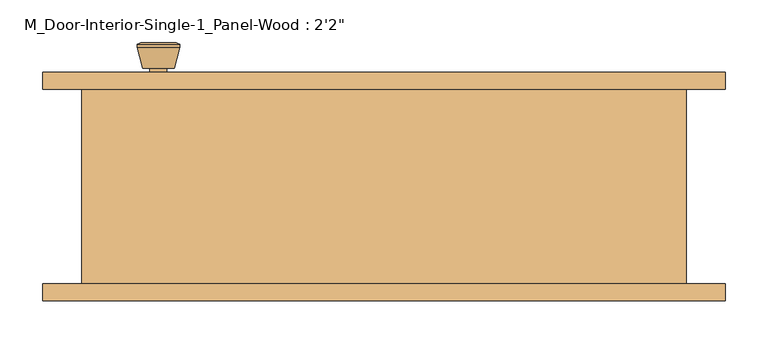
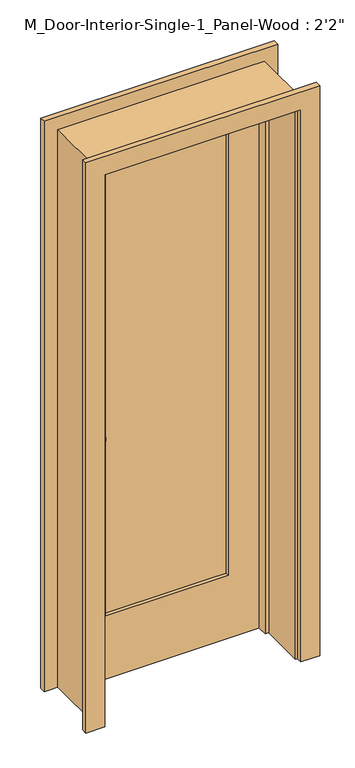
"""IFC4 building model written with IfcOpenShell, lengths in millimetres: door geometry."""

from ifc_helpers import new_model, si_unit, point, frame, frame_2d, origin, place, context, project, spatial, polyline, circle_curve, trimmed, segment, composite_curve, outline, extrude, faceted_brep, source, transform, mapped, element, save
from ifc_brep_helpers import plane_surface, cylinder_surface, revolved_surface, advanced_brep


def door_ae2d502c(model_context):
    return source(origin(), model_context, "Body", "SolidModel", [
        advanced_brep(
        [(-265.2, 70.125, 914.4), (-255.2, 70.125, 914.4), (-275.2, 70.125, 914.4), (-244.7241324, 21.125, 914.4), (-265.2, 21.125, 914.4), (-285.6758676, 21.125, 914.4), (-240.2, 22.9528681, 914.4), (-290.2, 22.9528681, 914.4), (-240.2, 26.4165463, 914.4), (-290.2, 26.4165463, 914.4), (-246.563764, 51.125, 914.4), (-283.836236, 51.125, 914.4), (-255.2, 51.125, 914.4), (-275.2, 51.125, 914.4)],
        [
            (0, 1),
            (1, 2, circle_curve(frame((-265.2, 70.125, 914.4), z_axis=(0.0, 1.0, 0.0), x_axis=(-1.0, 0.0, 0.0)), 10.0)),
            (2, 0),
            (2, 1, circle_curve(frame((-265.2, 70.125, 914.4), z_axis=(0.0, 1.0, 0.0), x_axis=(-1.0, 0.0, 0.0)), 10.0)),
            (3, 4),
            (4, 5),
            (5, 3, circle_curve(frame((-265.2, 21.125, 914.4), z_axis=(0.0, -1.0, 0.0), x_axis=(-1.0, 0.0, 0.0)), 20.4758676)),
            (3, 5, circle_curve(frame((-265.2, 21.125, 914.4), z_axis=(0.0, -1.0, 0.0), x_axis=(-1.0, 0.0, 0.0)), 20.4758676)),
            (6, 3),
            (5, 7),
            (7, 6, circle_curve(frame((-265.2, 22.9528681, 914.4), z_axis=(0.0, -1.0, 0.0), x_axis=(-1.0, 0.0, 0.0)), 25.0)),
            (6, 7, circle_curve(frame((-265.2, 22.9528681, 914.4), z_axis=(0.0, -1.0, 0.0), x_axis=(-1.0, 0.0, 0.0)), 25.0)),
            (8, 6),
            (7, 9),
            (9, 8, circle_curve(frame((-265.2, 26.4165463, 914.4), z_axis=(0.0, -1.0, 0.0), x_axis=(-1.0, 0.0, 0.0)), 25.0)),
            (8, 9, circle_curve(frame((-265.2, 26.4165463, 914.4), z_axis=(0.0, -1.0, 0.0), x_axis=(-1.0, 0.0, 0.0)), 25.0)),
            (10, 8),
            (9, 11),
            (11, 10, circle_curve(frame((-265.2, 51.125, 914.4), z_axis=(0.0, -1.0, 0.0), x_axis=(-1.0, 0.0, 0.0)), 18.636236)),
            (10, 11, circle_curve(frame((-265.2, 51.125, 914.4), z_axis=(0.0, -1.0, 0.0), x_axis=(-1.0, 0.0, 0.0)), 18.636236)),
            (12, 10),
            (11, 13),
            (13, 12, circle_curve(frame((-265.2, 51.125, 914.4), z_axis=(0.0, -1.0, 0.0), x_axis=(-1.0, 0.0, 0.0)), 10.0)),
            (12, 13, circle_curve(frame((-265.2, 51.125, 914.4), z_axis=(0.0, -1.0, 0.0), x_axis=(-1.0, 0.0, 0.0)), 10.0)),
            (1, 12),
            (13, 2),
        ],
        [
            plane_surface(frame((-265.2, 70.125, 914.4), z_axis=(0.0, 1.0, 0.0), x_axis=(-1.0, 0.0, 0.0))),
            plane_surface(frame((-265.2, 21.125, 914.4), z_axis=(0.0, -1.0, 0.0), x_axis=(-1.0, 0.0, 0.0))),
            revolved_surface(polyline([(-285.6758676, 21.125, 914.4), (-290.2, 22.9528681, 914.4)]), (-265.2, 70.125, 914.4), (0.0, 1.0, 0.0)),
            cylinder_surface(frame((-265.2, 70.125, 914.4), z_axis=(0.0, 1.0, 0.0), x_axis=(-1.0, 0.0, 0.0)), 25.0),
            revolved_surface(polyline([(-290.2, 26.4165463, 914.4), (-283.836236, 51.125, 914.4)]), (-265.2, 70.125, 914.4), (0.0, 1.0, 0.0)),
            plane_surface(frame((-265.2, 51.125, 914.4), z_axis=(0.0, 1.0, 0.0), x_axis=(-1.0, 0.0, 0.0))),
            cylinder_surface(frame((-265.2, 70.125, 914.4), z_axis=(0.0, 1.0, 0.0), x_axis=(-1.0, 0.0, 0.0)), 10.0),
        ],
        [
            (0, [[1, 2, 3]]),
            (0, [[-3, 4, -1]]),
            (1, [[5, 6, 7]]),
            (1, [[-6, -5, 8]]),
            (2, [[9, -7, 10, 11]]),
            (2, [[-10, -8, -9, 12]]),
            (3, [[13, -11, 14, 15]]),
            (3, [[-14, -12, -13, 16]]),
            (4, [[17, -15, 18, 19]]),
            (4, [[-18, -16, -17, 20]]),
            (5, [[21, -19, 22, 23]]),
            (5, [[-22, -20, -21, 24]]),
            (6, [[25, -23, 26, -2]]),
            (6, [[-26, -24, -25, -4]]),
        ],
    ),
        extrude(outline(composite_curve([segment(trimmed(circle_curve(frame_2d((914.4, -265.2)), 30.0), [point((914.4, -295.2))], [point((914.4, -235.2))], False, "CARTESIAN"), True, "CONTINUOUS"), segment(trimmed(circle_curve(frame_2d((914.4, -265.2)), 30.0), [point((914.4, -235.2))], [point((914.4, -295.2))], False, "CARTESIAN"), True, "CONTINUOUS")], self_intersect=False)), frame((0.0, 70.125, 0.0), z_axis=(0.0, 1.0, 0.0), x_axis=(0.0, 0.0, 1.0)), (0.0, 0.0, 1.0), 6.0),
        advanced_brep(
        [(-265.2, 117.125, 914.4), (-275.2, 117.125, 914.4), (-255.2, 117.125, 914.4), (-244.7241324, 166.125, 914.4), (-285.6758676, 166.125, 914.4), (-265.2, 166.125, 914.4), (-240.2, 164.2971319, 914.4), (-290.2, 164.2971319, 914.4), (-240.2, 160.8334537, 914.4), (-290.2, 160.8334537, 914.4), (-246.563764, 136.125, 914.4), (-283.836236, 136.125, 914.4), (-255.2, 136.125, 914.4), (-275.2, 136.125, 914.4)],
        [
            (0, 1),
            (1, 2, circle_curve(frame((-265.2, 117.125, 914.4), z_axis=(0.0, -1.0, 0.0), x_axis=(-1.0, 0.0, 0.0)), 10.0)),
            (2, 0),
            (2, 1, circle_curve(frame((-265.2, 117.125, 914.4), z_axis=(0.0, -1.0, 0.0), x_axis=(-1.0, 0.0, 0.0)), 10.0)),
            (3, 4, circle_curve(frame((-265.2, 166.125, 914.4), z_axis=(0.0, 1.0, 0.0), x_axis=(-1.0, 0.0, 0.0)), 20.4758676)),
            (4, 5),
            (5, 3),
            (4, 3, circle_curve(frame((-265.2, 166.125, 914.4), z_axis=(0.0, 1.0, 0.0), x_axis=(-1.0, 0.0, 0.0)), 20.4758676)),
            (6, 7, circle_curve(frame((-265.2, 164.2971319, 914.4), z_axis=(0.0, 1.0, 0.0), x_axis=(-1.0, 0.0, 0.0)), 25.0)),
            (7, 4),
            (3, 6),
            (7, 6, circle_curve(frame((-265.2, 164.2971319, 914.4), z_axis=(0.0, 1.0, 0.0), x_axis=(-1.0, 0.0, 0.0)), 25.0)),
            (8, 9, circle_curve(frame((-265.2, 160.8334537, 914.4), z_axis=(0.0, 1.0, 0.0), x_axis=(-1.0, 0.0, 0.0)), 25.0)),
            (9, 7),
            (6, 8),
            (9, 8, circle_curve(frame((-265.2, 160.8334537, 914.4), z_axis=(0.0, 1.0, 0.0), x_axis=(-1.0, 0.0, 0.0)), 25.0)),
            (10, 11, circle_curve(frame((-265.2, 136.125, 914.4), z_axis=(0.0, 1.0, 0.0), x_axis=(-1.0, 0.0, 0.0)), 18.636236)),
            (11, 9),
            (8, 10),
            (11, 10, circle_curve(frame((-265.2, 136.125, 914.4), z_axis=(0.0, 1.0, 0.0), x_axis=(-1.0, 0.0, 0.0)), 18.636236)),
            (12, 13, circle_curve(frame((-265.2, 136.125, 914.4), z_axis=(0.0, 1.0, 0.0), x_axis=(-1.0, 0.0, 0.0)), 10.0)),
            (13, 11),
            (10, 12),
            (13, 12, circle_curve(frame((-265.2, 136.125, 914.4), z_axis=(0.0, 1.0, 0.0), x_axis=(-1.0, 0.0, 0.0)), 10.0)),
            (1, 13),
            (12, 2),
        ],
        [
            plane_surface(frame((-265.2, 117.125, 914.4), z_axis=(0.0, -1.0, 0.0), x_axis=(-1.0, 0.0, 0.0))),
            plane_surface(frame((-265.2, 166.125, 914.4), z_axis=(0.0, 1.0, 0.0), x_axis=(-1.0, 0.0, 0.0))),
            revolved_surface(polyline([(-285.6758676, 166.125, 914.4), (-290.2, 164.2971319, 914.4)]), (-265.2, 117.125, 914.4), (0.0, -1.0, 0.0)),
            cylinder_surface(frame((-265.2, 117.125, 914.4), z_axis=(0.0, -1.0, 0.0), x_axis=(-1.0, 0.0, 0.0)), 25.0),
            revolved_surface(polyline([(-290.2, 160.8334537, 914.4), (-283.836236, 136.125, 914.4)]), (-265.2, 117.125, 914.4), (0.0, -1.0, 0.0)),
            plane_surface(frame((-265.2, 136.125, 914.4), z_axis=(0.0, -1.0, 0.0), x_axis=(-1.0, 0.0, 0.0))),
            cylinder_surface(frame((-265.2, 117.125, 914.4), z_axis=(0.0, -1.0, 0.0), x_axis=(-1.0, 0.0, 0.0)), 10.0),
        ],
        [
            (0, [[1, 2, 3]]),
            (0, [[-3, 4, -1]]),
            (1, [[5, 6, 7]]),
            (1, [[8, -7, -6]]),
            (2, [[9, 10, -5, 11]]),
            (2, [[12, -11, -8, -10]]),
            (3, [[13, 14, -9, 15]]),
            (3, [[16, -15, -12, -14]]),
            (4, [[17, 18, -13, 19]]),
            (4, [[20, -19, -16, -18]]),
            (5, [[21, 22, -17, 23]]),
            (5, [[24, -23, -20, -22]]),
            (6, [[-2, 25, -21, 26]]),
            (6, [[-4, -26, -24, -25]]),
        ],
    ),
        extrude(outline(composite_curve([segment(trimmed(circle_curve(frame_2d((914.4, -265.2)), 30.0), [point((914.4, -295.2))], [point((914.4, -235.2))], False, "CARTESIAN"), True, "CONTINUOUS"), segment(trimmed(circle_curve(frame_2d((914.4, -265.2)), 30.0), [point((914.4, -235.2))], [point((914.4, -295.2))], False, "CARTESIAN"), True, "CONTINUOUS")], self_intersect=False)), frame((0.0, 111.125, 0.0), z_axis=(0.0, 1.0, 0.0), x_axis=(0.0, 0.0, 1.0)), (0.0, 0.0, 1.0), 6.0),
        faceted_brep([(355.2, 111.125, 0.0), (355.2, -117.475, 0.0), (330.2, -117.475, 0.0), (330.2, 41.2, 0.0), (317.5, 41.2, 0.0), (317.5, 76.125, 0.0), (330.2, 76.125, 0.0), (330.2, 111.125, 0.0), (355.2, 111.125, 2025.0), (355.2, -117.475, 2025.0), (-355.2, -117.475, 2025.0), (-355.2, -117.475, 0.0), (-330.2, -117.475, 0.0), (-330.2, -117.475, 2000.0), (330.2, -117.475, 2000.0), (330.2, 41.2, 2000.0), (-330.2, 41.2, 2000.0), (-330.2, 41.2, 0.0), (-317.5, 41.2, 0.0), (-317.5, 41.2, 1987.3), (317.5, 41.2, 1987.3), (317.5, 76.125, 1987.3), (-317.5, 76.125, 1987.3), (-317.5, 76.125, 0.0), (-330.2, 76.125, 0.0), (-330.2, 76.125, 2000.0), (330.2, 76.125, 2000.0), (330.2, 111.125, 2000.0), (-330.2, 111.125, 2000.0), (-330.2, 111.125, 0.0), (-355.2, 111.125, 0.0), (-355.2, 111.125, 2025.0)], [[[0, 1, 2, 3, 4, 5, 6, 7]], [[1, 0, 8, 9]], [[2, 1, 9, 10, 11, 12, 13, 14]], [[3, 2, 14, 15]], [[4, 3, 15, 16, 17, 18, 19, 20]], [[5, 4, 20, 21]], [[6, 5, 21, 22, 23, 24, 25, 26]], [[7, 6, 26, 27]], [[0, 7, 27, 28, 29, 30, 31, 8]], [[9, 8, 31, 10]], [[15, 14, 13, 16]], [[21, 20, 19, 22]], [[27, 26, 25, 28]], [[30, 29, 24, 23, 18, 17, 12, 11]], [[10, 31, 30, 11]], [[16, 13, 12, 17]], [[22, 19, 18, 23]], [[28, 25, 24, 29]]]),
        extrude(outline(polyline([(2000.0, -330.2), (0.0, -330.2), (0.0, 330.2), (2000.0, 330.2), (2000.0, -330.2)]), holes=[polyline([(1880.0, -210.2), (1880.0, 210.2), (230.0, 210.2), (230.0, -210.2), (1880.0, -210.2)])]), frame((0.0, 76.125, 0.0), z_axis=(0.0, 1.0, 0.0), x_axis=(0.0, 0.0, 1.0)), (0.0, 0.0, 1.0), 35.0),
        extrude(outline(polyline([(210.2, 87.7916667), (-210.2, 87.7916667), (-210.2, 99.4583333), (210.2, 99.4583333), (210.2, 87.7916667)])), frame((0.0, 0.0, 230.0), z_axis=(0.0, 0.0, 1.0), x_axis=(1.0, 0.0, 0.0)), (0.0, 0.0, 1.0), 1650.0),
        extrude(outline(polyline([(0.0, 336.55), (0.0, 401.55), (2071.35, 401.55), (2071.35, -401.55), (0.0, -401.55), (0.0, -336.55), (2006.35, -336.55), (2006.35, 336.55), (0.0, 336.55)])), frame((0.0, 111.125, 0.0), z_axis=(0.0, 1.0, 0.0), x_axis=(0.0, 0.0, 1.0)), (0.0, 0.0, 1.0), 20.0),
        extrude(outline(polyline([(0.0, 336.55), (0.0, 401.55), (2071.35, 401.55), (2071.35, -401.55), (0.0, -401.55), (0.0, -336.55), (2006.35, -336.55), (2006.35, 336.55), (0.0, 336.55)])), frame((0.0, -137.475, 0.0), z_axis=(0.0, 1.0, 0.0), x_axis=(0.0, 0.0, 1.0)), (0.0, 0.0, 1.0), 20.0),
    ])


if __name__ == "__main__":
    model = new_model("IFC4")
    model_context = context("Model", 3, world=origin())
    ifc_project = project(units=[si_unit("LENGTHUNIT", "METRE", prefix="MILLI")], contexts=[model_context])
    site = spatial("IfcSite", under=ifc_project)
    building = spatial("IfcBuilding", under=site)
    placement = place(None, origin())
    door_shape = door_ae2d502c(model_context)
    element("IfcDoor", 1, ObjectType="M_Door-Interior-Single-1_Panel-Wood : 2'2\"", at=placement, inside=building, context=model_context, shape_type="MappedRepresentation", body=[
        mapped(door_shape, transform((0.0, 0.0, 0.0), x_axis=(1.0, 0.0, 0.0), y_axis=(0.0, 1.0, 0.0), z_axis=(0.0, 0.0, 1.0))),
    ])
    save(model, "model.ifc")

# Revit data of these elements
# Type "M_Door-Interior-Single-1_Panel-Wood : 2'2\""
#   Type Mark = "17"
#   Assembly Code = "C1020300"
#   Analytic Construction = "Wooden"
#   Top Rail = 0' - 4.72441"
#   Thickness = 0' - 1.37795"
#   Thermal Resistance (R) = 2.5876 (h·ft²·°F)/BTU
#   Swing Angle [instance default] = 90.00°
#   Stiles = 0' - 4.72441"
#   Rough Width = 2' - 3.9685"
#   Rough Height = 6' - 7.72441"
#   Height = 6' - 6.74016"
#   Width = 2' - 2"
#   Heat Transfer Coefficient (U) = 0.3865 BTU/(h·ft²·°F)
#   Bottom Rail = 0' - 9.05512"
#   Trim Material = Cherry
#   Panel Material = Cherry
#   Frame Material = Cherry
#   Door Handle Material = Aluminum
#   Visual Light Transmittance = 0
#   Solar Heat Gain Coefficient = 0
#   Wall Closure = (empty or 0)
#   Function = (empty or 0)
# Element 1 (IfcDoor, "M_Door-Interior-Single-1_Panel-Wood : 2'2\"")
#   Materials on its faces: "Cherry", "Aluminum"
# Materials
#   "Cherry": class "Wood", colour RGB 226 177 128, transparency 0, Description = "Prunus Serotina", Cost = 0
#   "Aluminum": class "Metal", colour RGB 247 247 247, transparency 0, Description = "Aluminum 6061", Cost = 0
